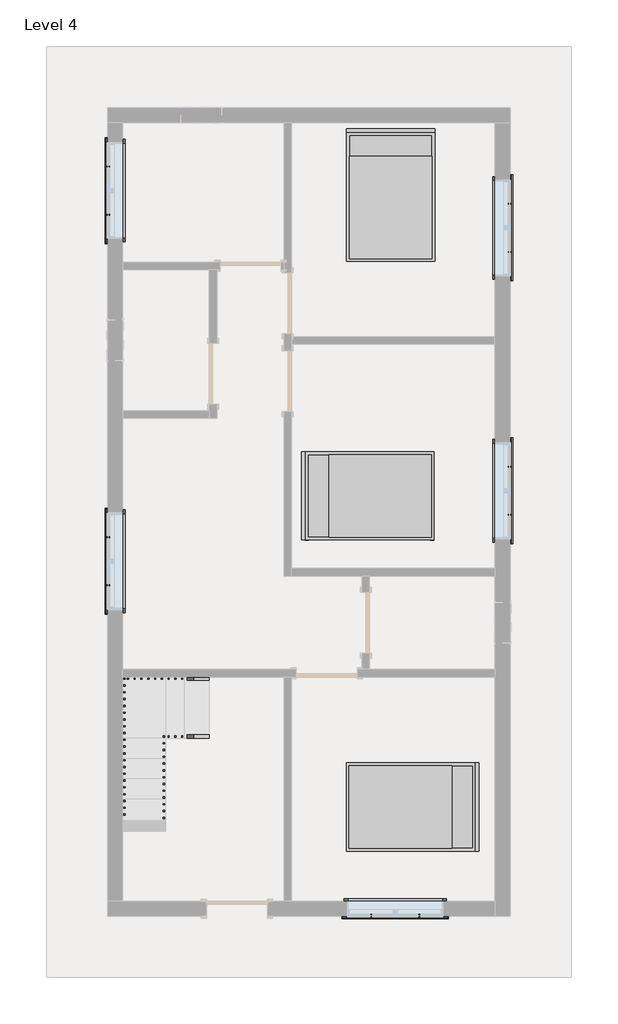
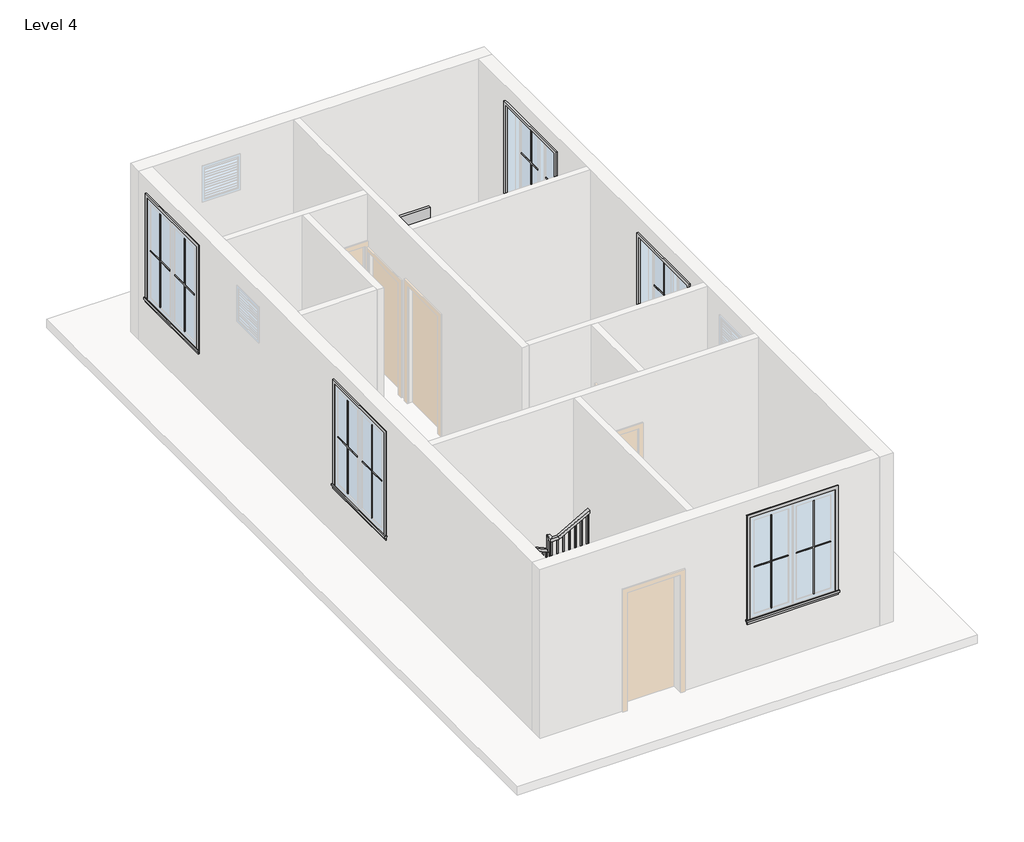
# One storey, part 2 of 2: 20 proxies, 3 furniture elements, 2 railings.
"""IFC4 building model written with IfcOpenShell, lengths in millimetres."""

from ifc_helpers import new_model, si_unit, frame, origin, place, context, project, spatial, polyline, outline, extrude, faceted_brep, transform, mapped, element, save
from components import muntin_pattern_2x2_muntin_pattern_2x2_bff912c5, muntin_pattern_2x2_muntin_pattern_2x2_c2194282, trim_window_exterior_flat_with_sill_e04b3088, trim_window_interior_flat_picture_frame_2a7685fe, bed_17739_bed_17739_15c61121

model = new_model("IFC4")

# Units and contexts
model_context = context("Model", 3, world=origin())
ifc_project = project(units=[si_unit("LENGTHUNIT", "METRE", prefix="MILLI")], contexts=[model_context])

# Site, building, storey
site = spatial("IfcSite", under=ifc_project)
building = spatial("IfcBuilding", under=site)
storey = spatial("IfcBuildingStorey", under=building, Name="Level 4", Elevation=6400.8)

# Proxies
placement = place(None, origin())
muntin_pattern_2x2_muntin_pattern_2x2_shape = muntin_pattern_2x2_muntin_pattern_2x2_bff912c5(model_context)
element("IfcBuildingElementProxy", 1, Name="Muntin Pattern_2x2 : Muntin Pattern_2x2", ObjectType="Muntin Pattern_2x2 : Muntin Pattern_2x2", at=placement, inside=storey, context=model_context, shape_type="MappedRepresentation", body=[
    mapped(muntin_pattern_2x2_muntin_pattern_2x2_shape, transform((-4261.9639285, 4584.2694249, 7385.05), x_axis=(0.0, 1.0, 0.0), y_axis=(-1.0, 0.0, 0.0), z_axis=(0.0, 0.0, 1.0))),
])
element("IfcBuildingElementProxy", 2, Name="Muntin Pattern_2x2 : Muntin Pattern_2x2", ObjectType="Muntin Pattern_2x2 : Muntin Pattern_2x2", at=placement, inside=storey, context=model_context, shape_type="MappedRepresentation", body=[
    mapped(muntin_pattern_2x2_muntin_pattern_2x2_shape, transform((1751.4860715, 4746.1944249, 7385.05), x_axis=(0.0, -1.0, 0.0), y_axis=(1.0, 0.0, 0.0), z_axis=(0.0, 0.0, 1.0))),
])
element("IfcBuildingElementProxy", 3, Name="Muntin Pattern_2x2 : Muntin Pattern_2x2", ObjectType="Muntin Pattern_2x2 : Muntin Pattern_2x2", at=placement, inside=storey, context=model_context, shape_type="MappedRepresentation", body=[
    mapped(muntin_pattern_2x2_muntin_pattern_2x2_shape, transform((-4261.9639285, -962.4555751, 7385.05), x_axis=(0.0, 1.0, 0.0), y_axis=(-1.0, 0.0, 0.0), z_axis=(0.0, 0.0, 1.0))),
])
element("IfcBuildingElementProxy", 4, Name="Muntin Pattern_2x2 : Muntin Pattern_2x2", ObjectType="Muntin Pattern_2x2 : Muntin Pattern_2x2", at=placement, inside=storey, context=model_context, shape_type="MappedRepresentation", body=[
    mapped(muntin_pattern_2x2_muntin_pattern_2x2_shape, transform((1751.4860715, 812.3694249, 7385.05), x_axis=(0.0, -1.0, 0.0), y_axis=(1.0, 0.0, 0.0), z_axis=(0.0, 0.0, 1.0))),
])
element("IfcBuildingElementProxy", 5, Name="Muntin Pattern_2x2 : Muntin Pattern_2x2", ObjectType="Muntin Pattern_2x2 : Muntin Pattern_2x2", at=placement, inside=storey, context=model_context, shape_type="MappedRepresentation", body=[
    mapped(muntin_pattern_2x2_muntin_pattern_2x2_shape, transform((397.3485715, -5907.5180751, 7385.05), x_axis=(-1.0, 0.0, 0.0), y_axis=(0.0, -1.0, 0.0), z_axis=(0.0, 0.0, 1.0))),
])
muntin_pattern_2x2_muntin_pattern_2x2_2_shape = muntin_pattern_2x2_muntin_pattern_2x2_c2194282(model_context)
element("IfcBuildingElementProxy", 6, Name="Muntin Pattern_2x2 : Muntin Pattern_2x2", ObjectType="Muntin Pattern_2x2 : Muntin Pattern_2x2", at=placement, inside=storey, context=model_context, shape_type="MappedRepresentation", body=[
    mapped(muntin_pattern_2x2_muntin_pattern_2x2_2_shape, transform((-4261.9639285, 5304.9944249, 7385.05), x_axis=(0.0, -1.0, 0.0), y_axis=(1.0, 0.0, 0.0), z_axis=(0.0, 0.0, 1.0))),
])
element("IfcBuildingElementProxy", 7, Name="Muntin Pattern_2x2 : Muntin Pattern_2x2", ObjectType="Muntin Pattern_2x2 : Muntin Pattern_2x2", at=placement, inside=storey, context=model_context, shape_type="MappedRepresentation", body=[
    mapped(muntin_pattern_2x2_muntin_pattern_2x2_2_shape, transform((1751.4860715, 4025.4694249, 7385.05), x_axis=(0.0, 1.0, 0.0), y_axis=(-1.0, 0.0, 0.0), z_axis=(0.0, 0.0, 1.0))),
])
element("IfcBuildingElementProxy", 8, Name="Muntin Pattern_2x2 : Muntin Pattern_2x2", ObjectType="Muntin Pattern_2x2 : Muntin Pattern_2x2", at=placement, inside=storey, context=model_context, shape_type="MappedRepresentation", body=[
    mapped(muntin_pattern_2x2_muntin_pattern_2x2_2_shape, transform((-4261.9639285, -241.7305751, 7385.05), x_axis=(0.0, -1.0, 0.0), y_axis=(1.0, 0.0, 0.0), z_axis=(0.0, 0.0, 1.0))),
])
element("IfcBuildingElementProxy", 9, Name="Muntin Pattern_2x2 : Muntin Pattern_2x2", ObjectType="Muntin Pattern_2x2 : Muntin Pattern_2x2", at=placement, inside=storey, context=model_context, shape_type="MappedRepresentation", body=[
    mapped(muntin_pattern_2x2_muntin_pattern_2x2_2_shape, transform((1751.4860715, 91.6444249, 7385.05), x_axis=(0.0, 1.0, 0.0), y_axis=(-1.0, 0.0, 0.0), z_axis=(0.0, 0.0, 1.0))),
])
element("IfcBuildingElementProxy", 10, Name="Muntin Pattern_2x2 : Muntin Pattern_2x2", ObjectType="Muntin Pattern_2x2 : Muntin Pattern_2x2", at=placement, inside=storey, context=model_context, shape_type="MappedRepresentation", body=[
    mapped(muntin_pattern_2x2_muntin_pattern_2x2_2_shape, transform((-323.3764285, -5907.5180751, 7385.05), x_axis=(1.0, 0.0, 0.0), y_axis=(0.0, 1.0, 0.0), z_axis=(0.0, 0.0, 1.0))),
])
trim_window_exterior_flat_with_sill_shape = trim_window_exterior_flat_with_sill_e04b3088(model_context)
element("IfcBuildingElementProxy", 11, Name="Trim-Window-Exterior-Flat : with Sill", ObjectType="Trim-Window-Exterior-Flat : with Sill", at=placement, inside=storey, context=model_context, shape_type="MappedRepresentation", body=[
    mapped(trim_window_exterior_flat_with_sill_shape, transform((-4271.4889285, 4944.6319249, 9144.0), x_axis=(0.0, -1.0, 0.0), y_axis=(0.0, 0.0, 1.0), z_axis=(-1.0, 0.0, 0.0))),
])
element("IfcBuildingElementProxy", 12, Name="Trim-Window-Exterior-Flat : with Sill", ObjectType="Trim-Window-Exterior-Flat : with Sill", at=placement, inside=storey, context=model_context, shape_type="MappedRepresentation", body=[
    mapped(trim_window_exterior_flat_with_sill_shape, transform((1761.0110715, 4385.8319249, 9144.0), x_axis=(0.0, 1.0, 0.0), y_axis=(0.0, 0.0, 1.0), z_axis=(1.0, 0.0, 0.0))),
])
element("IfcBuildingElementProxy", 13, Name="Trim-Window-Exterior-Flat : with Sill", ObjectType="Trim-Window-Exterior-Flat : with Sill", at=placement, inside=storey, context=model_context, shape_type="MappedRepresentation", body=[
    mapped(trim_window_exterior_flat_with_sill_shape, transform((-4271.4889285, -602.0930751, 9144.0), x_axis=(0.0, -1.0, 0.0), y_axis=(0.0, 0.0, 1.0), z_axis=(-1.0, 0.0, 0.0))),
])
element("IfcBuildingElementProxy", 14, Name="Trim-Window-Exterior-Flat : with Sill", ObjectType="Trim-Window-Exterior-Flat : with Sill", at=placement, inside=storey, context=model_context, shape_type="MappedRepresentation", body=[
    mapped(trim_window_exterior_flat_with_sill_shape, transform((1761.0110715, 452.0069249, 9144.0), x_axis=(0.0, 1.0, 0.0), y_axis=(0.0, 0.0, 1.0), z_axis=(1.0, 0.0, 0.0))),
])
element("IfcBuildingElementProxy", 15, Name="Trim-Window-Exterior-Flat : with Sill", ObjectType="Trim-Window-Exterior-Flat : with Sill", at=placement, inside=storey, context=model_context, shape_type="MappedRepresentation", body=[
    mapped(trim_window_exterior_flat_with_sill_shape, transform((36.9860715, -5917.0430751, 9144.0), x_axis=(1.0, 0.0, 0.0), y_axis=(0.0, 0.0, 1.0), z_axis=(0.0, -1.0, 0.0))),
])
trim_window_interior_flat_picture_frame_shape = trim_window_interior_flat_picture_frame_2a7685fe(model_context)
element("IfcBuildingElementProxy", 16, Name="Trim-Window-Interior-Flat : Picture Frame", ObjectType="Trim-Window-Interior-Flat : Picture Frame", at=placement, inside=storey, context=model_context, shape_type="MappedRepresentation", body=[
    mapped(trim_window_interior_flat_picture_frame_shape, transform((-4042.8889285, 4944.6319249, 9144.0), x_axis=(0.0, 1.0, 0.0), y_axis=(0.0, 0.0, 1.0), z_axis=(1.0, 0.0, 0.0))),
])
element("IfcBuildingElementProxy", 17, Name="Trim-Window-Interior-Flat : Picture Frame", ObjectType="Trim-Window-Interior-Flat : Picture Frame", at=placement, inside=storey, context=model_context, shape_type="MappedRepresentation", body=[
    mapped(trim_window_interior_flat_picture_frame_shape, transform((1532.4110715, 4385.8319249, 9144.0), x_axis=(0.0, -1.0, 0.0), y_axis=(0.0, 0.0, 1.0), z_axis=(-1.0, 0.0, 0.0))),
])
element("IfcBuildingElementProxy", 18, Name="Trim-Window-Interior-Flat : Picture Frame", ObjectType="Trim-Window-Interior-Flat : Picture Frame", at=placement, inside=storey, context=model_context, shape_type="MappedRepresentation", body=[
    mapped(trim_window_interior_flat_picture_frame_shape, transform((-4042.8889285, -602.0930751, 9144.0), x_axis=(0.0, 1.0, 0.0), y_axis=(0.0, 0.0, 1.0), z_axis=(1.0, 0.0, 0.0))),
])
element("IfcBuildingElementProxy", 19, Name="Trim-Window-Interior-Flat : Picture Frame", ObjectType="Trim-Window-Interior-Flat : Picture Frame", at=placement, inside=storey, context=model_context, shape_type="MappedRepresentation", body=[
    mapped(trim_window_interior_flat_picture_frame_shape, transform((1532.4110715, 452.0069249, 9144.0), x_axis=(0.0, -1.0, 0.0), y_axis=(0.0, 0.0, 1.0), z_axis=(-1.0, 0.0, 0.0))),
])
element("IfcBuildingElementProxy", 20, Name="Trim-Window-Interior-Flat : Picture Frame", ObjectType="Trim-Window-Interior-Flat : Picture Frame", at=placement, inside=storey, context=model_context, shape_type="MappedRepresentation", body=[
    mapped(trim_window_interior_flat_picture_frame_shape, transform((36.9860715, -5688.4430751, 9144.0), x_axis=(-1.0, 0.0, 0.0), y_axis=(0.0, 0.0, 1.0), z_axis=(0.0, 1.0, 0.0))),
])

# Furniture
bed_17739_bed_17739_shape = bed_17739_bed_17739_15c61121(model_context)
element("IfcFurniture", 21, ObjectType="Bed_17739 : Bed_17739", at=placement, inside=storey, context=model_context, shape_type="MappedRepresentation", body=[
    mapped(bed_17739_bed_17739_shape, transform((-29.6889285, 4852.5569249, 6400.8), x_axis=(1.0, 0.0, 0.0), y_axis=(0.0, 1.0, 0.0), z_axis=(0.0, 0.0, 1.0))),
])
element("IfcFurniture", 22, ObjectType="Bed_17739 : Bed_17739", at=placement, inside=storey, context=model_context, shape_type="MappedRepresentation", body=[
    mapped(bed_17739_bed_17739_shape, transform((-347.1889285, 375.8069249, 6400.8), x_axis=(0.0, 1.0, 0.0), y_axis=(-1.0, 0.0, 0.0), z_axis=(0.0, 0.0, 1.0))),
])
element("IfcFurniture", 23, ObjectType="Bed_17739 : Bed_17739", at=placement, inside=storey, context=model_context, shape_type="MappedRepresentation", body=[
    mapped(bed_17739_bed_17739_shape, transform((275.1110715, -4278.7430751, 6400.8), x_axis=(0.0, -1.0, 0.0), y_axis=(1.0, 0.0, 0.0), z_axis=(0.0, 0.0, 1.0))),
])

# Railings
element("IfcRailing", 24, ObjectType="Handrail - Rectangular", at=placement, inside=storey, context=model_context, shape_type="SolidModel", body=[
    faceted_brep([(-2747.4889285, -2386.4430751, 7484.5333333), (-2747.4889285, -2386.4430751, 7427.3271159), (-2747.4889285, -2335.6430751, 7427.3271159), (-2747.4889285, -2335.6430751, 7484.5333333), (-3396.0267484, -2386.4430751, 7820.3457967), (-3408.3987558, -2386.4430751, 7769.5457967), (-3408.3987558, -2335.6430751, 7769.5457967), (-3396.0267484, -2335.6430751, 7820.3457967), (-3992.0889285, -2386.4430751, 7820.3457967), (-3992.0889285, -2386.4430751, 7769.5457967), (-4042.8889285, -2335.6430751, 7769.5457967), (-4042.8889285, -2335.6430751, 7820.3457967), (-3992.0889285, -2940.1628326, 7820.3457967), (-3992.0889285, -2953.3285634, 7769.5457967), (-4042.8889285, -2953.3285634, 7769.5457967), (-4042.8889285, -2940.1628326, 7820.3457967), (-3992.0889285, -5061.9991591, 8999.3618165), (-3992.0889285, -5075.1648899, 8948.5618165), (-4042.8889285, -5075.1648899, 8948.5618165), (-4042.8889285, -5061.9991591, 8999.3618165), (-3992.0889285, -5637.6430751, 8999.3618165), (-3992.0889285, -5637.6430751, 8948.5618165), (-4042.8889285, -5688.4430751, 8948.5618165), (-4042.8889285, -5688.4430751, 8999.3618165), (-3418.001852, -5637.6430751, 8999.3618165), (-3404.8062484, -5637.6430751, 8948.5618165), (-3404.8062484, -5688.4430751, 8948.5618165), (-3418.001852, -5688.4430751, 8999.3618165), (-2793.6303845, -5637.6430751, 9347.2), (-2793.6303845, -5688.4430751, 9347.2), (-2793.6303845, -5688.4430751, 9289.0487115), (-2793.6303845, -5637.6430751, 9289.0487115)], [[[0, 1, 2, 3]], [[1, 0, 4, 5]], [[2, 1, 5, 6]], [[3, 2, 6, 7]], [[0, 3, 7, 4]], [[5, 4, 8, 9]], [[6, 5, 9, 10]], [[7, 6, 10, 11]], [[4, 7, 11, 8]], [[9, 8, 12, 13]], [[10, 9, 13, 14]], [[11, 10, 14, 15]], [[8, 11, 15, 12]], [[13, 12, 16, 17]], [[14, 13, 17, 18]], [[15, 14, 18, 19]], [[12, 15, 19, 16]], [[17, 16, 20, 21]], [[18, 17, 21, 22]], [[19, 18, 22, 23]], [[16, 19, 23, 20]], [[21, 20, 24, 25]], [[22, 21, 25, 26]], [[23, 22, 26, 27]], [[20, 23, 27, 24]], [[28, 29, 30, 31]], [[25, 24, 28, 31]], [[26, 25, 31, 30]], [[27, 26, 30, 29]], [[24, 27, 29, 28]]]),
    extrude(outline(polyline([(9291.7598207, -2788.7639285), (9281.1470401, -2807.8139285), (8263.4666667, -2807.8139285), (8263.4666667, -2788.7639285), (9291.7598207, -2788.7639285)])), frame((0.0, -5672.5680751, 0.0), z_axis=(0.0, 1.0, 0.0), x_axis=(0.0, 0.0, 1.0)), (0.0, 0.0, 1.0), 19.05),
    extrude(outline(polyline([(9235.1583242, -2890.3639285), (9224.5455436, -2909.4139285), (8263.4666667, -2909.4139285), (8263.4666667, -2890.3639285), (9235.1583242, -2890.3639285)])), frame((0.0, -5672.5680751, 0.0), z_axis=(0.0, 1.0, 0.0), x_axis=(0.0, 0.0, 1.0)), (0.0, 0.0, 1.0), 19.05),
    extrude(outline(polyline([(9178.5568277, -2991.9639285), (9167.9440471, -3011.0139285), (8263.4666667, -3011.0139285), (8263.4666667, -2991.9639285), (9178.5568277, -2991.9639285)])), frame((0.0, -5672.5680751, 0.0), z_axis=(0.0, 1.0, 0.0), x_axis=(0.0, 0.0, 1.0)), (0.0, 0.0, 1.0), 19.05),
    extrude(outline(polyline([(9121.9553312, -3093.5639285), (9111.3425506, -3112.6139285), (8263.4666667, -3112.6139285), (8263.4666667, -3093.5639285), (9121.9553312, -3093.5639285)])), frame((0.0, -5672.5680751, 0.0), z_axis=(0.0, 1.0, 0.0), x_axis=(0.0, 0.0, 1.0)), (0.0, 0.0, 1.0), 19.05),
    extrude(outline(polyline([(9065.3538346, -3195.1639285), (9054.7410541, -3214.2139285), (8094.1333333, -3214.2139285), (8094.1333333, -3195.1639285), (9065.3538346, -3195.1639285)])), frame((0.0, -5672.5680751, 0.0), z_axis=(0.0, 1.0, 0.0), x_axis=(0.0, 0.0, 1.0)), (0.0, 0.0, 1.0), 19.05),
    extrude(outline(polyline([(9008.7523381, -3296.7639285), (8998.1395575, -3315.8139285), (8094.1333333, -3315.8139285), (8094.1333333, -3296.7639285), (9008.7523381, -3296.7639285)])), frame((0.0, -5672.5680751, 0.0), z_axis=(0.0, 1.0, 0.0), x_axis=(0.0, 0.0, 1.0)), (0.0, 0.0, 1.0), 19.05),
    extrude(outline(polyline([(8952.1508416, -3398.3639285), (8941.538061, -3417.4139285), (7924.8, -3417.4139285), (7924.8, -3398.3639285), (8952.1508416, -3398.3639285)])), frame((0.0, -5672.5680751, 0.0), z_axis=(0.0, 1.0, 0.0), x_axis=(0.0, 0.0, 1.0)), (0.0, 0.0, 1.0), 19.05),
    extrude(outline(polyline([(-3519.0139285, -5672.5680751), (-3519.0139285, -5653.5180751), (-3499.9639285, -5653.5180751), (-3499.9639285, -5672.5680751), (-3519.0139285, -5672.5680751)])), frame((0.0, 0.0, 7924.8), z_axis=(0.0, 0.0, 1.0), x_axis=(1.0, 0.0, 0.0)), (0.0, 0.0, 1.0), 1023.7618165),
    extrude(outline(polyline([(-3620.6139285, -5672.5680751), (-3620.6139285, -5653.5180751), (-3601.5639285, -5653.5180751), (-3601.5639285, -5672.5680751), (-3620.6139285, -5672.5680751)])), frame((0.0, 0.0, 7924.8), z_axis=(0.0, 0.0, 1.0), x_axis=(1.0, 0.0, 0.0)), (0.0, 0.0, 1.0), 1023.7618165),
    extrude(outline(polyline([(-3722.2139285, -5672.5680751), (-3722.2139285, -5653.5180751), (-3703.1639285, -5653.5180751), (-3703.1639285, -5672.5680751), (-3722.2139285, -5672.5680751)])), frame((0.0, 0.0, 7924.8), z_axis=(0.0, 0.0, 1.0), x_axis=(1.0, 0.0, 0.0)), (0.0, 0.0, 1.0), 1023.7618165),
    extrude(outline(polyline([(-3823.8139285, -5672.5680751), (-3823.8139285, -5653.5180751), (-3804.7639285, -5653.5180751), (-3804.7639285, -5672.5680751), (-3823.8139285, -5672.5680751)])), frame((0.0, 0.0, 7924.8), z_axis=(0.0, 0.0, 1.0), x_axis=(1.0, 0.0, 0.0)), (0.0, 0.0, 1.0), 1023.7618165),
    extrude(outline(polyline([(-3925.4139285, -5672.5680751), (-3925.4139285, -5653.5180751), (-3906.3639285, -5653.5180751), (-3906.3639285, -5672.5680751), (-3925.4139285, -5672.5680751)])), frame((0.0, 0.0, 7924.8), z_axis=(0.0, 0.0, 1.0), x_axis=(1.0, 0.0, 0.0)), (0.0, 0.0, 1.0), 1023.7618165),
    extrude(outline(polyline([(-4027.0139285, -5602.7180751), (-4007.9639285, -5602.7180751), (-4007.9639285, -5621.7680751), (-4027.0139285, -5621.7680751), (-4027.0139285, -5602.7180751)])), frame((0.0, 0.0, 7924.8), z_axis=(0.0, 0.0, 1.0), x_axis=(1.0, 0.0, 0.0)), (0.0, 0.0, 1.0), 1023.7618165),
    extrude(outline(polyline([(-4027.0139285, -5501.1180751), (-4007.9639285, -5501.1180751), (-4007.9639285, -5520.1680751), (-4027.0139285, -5520.1680751), (-4027.0139285, -5501.1180751)])), frame((0.0, 0.0, 7924.8), z_axis=(0.0, 0.0, 1.0), x_axis=(1.0, 0.0, 0.0)), (0.0, 0.0, 1.0), 1023.7618165),
    extrude(outline(polyline([(-4027.0139285, -5399.5180751), (-4007.9639285, -5399.5180751), (-4007.9639285, -5418.5680751), (-4027.0139285, -5418.5680751), (-4027.0139285, -5399.5180751)])), frame((0.0, 0.0, 7924.8), z_axis=(0.0, 0.0, 1.0), x_axis=(1.0, 0.0, 0.0)), (0.0, 0.0, 1.0), 1023.7618165),
    extrude(outline(polyline([(-4027.0139285, -5297.9180751), (-4007.9639285, -5297.9180751), (-4007.9639285, -5316.9680751), (-4027.0139285, -5316.9680751), (-4027.0139285, -5297.9180751)])), frame((0.0, 0.0, 7924.8), z_axis=(0.0, 0.0, 1.0), x_axis=(1.0, 0.0, 0.0)), (0.0, 0.0, 1.0), 1023.7618165),
    extrude(outline(polyline([(-4027.0139285, -5196.3180751), (-4007.9639285, -5196.3180751), (-4007.9639285, -5215.3680751), (-4027.0139285, -5215.3680751), (-4027.0139285, -5196.3180751)])), frame((0.0, 0.0, 7924.8), z_axis=(0.0, 0.0, 1.0), x_axis=(1.0, 0.0, 0.0)), (0.0, 0.0, 1.0), 1023.7618165),
    extrude(outline(polyline([(-4027.0139285, -5094.7180751), (-4007.9639285, -5094.7180751), (-4007.9639285, -5113.7680751), (-4027.0139285, -5113.7680751), (-4027.0139285, -5094.7180751)])), frame((0.0, 0.0, 7924.8), z_axis=(0.0, 0.0, 1.0), x_axis=(1.0, 0.0, 0.0)), (0.0, 0.0, 1.0), 1023.7618165),
    extrude(outline(polyline([(-5012.1680751, 8913.5571119), (-4993.1180751, 8902.9718208), (-4993.1180751, 7924.8), (-5012.1680751, 7924.8), (-5012.1680751, 8913.5571119)])), frame((-4027.0139285, 0.0, 0.0), z_axis=(1.0, 0.0, 0.0), x_axis=(0.0, 1.0, 0.0)), (0.0, 0.0, 1.0), 19.05),
    extrude(outline(polyline([(-4910.5680751, 8857.1022261), (-4891.5180751, 8846.516935), (-4891.5180751, 7924.8), (-4910.5680751, 7924.8), (-4910.5680751, 8857.1022261)])), frame((-4027.0139285, 0.0, 0.0), z_axis=(1.0, 0.0, 0.0), x_axis=(0.0, 1.0, 0.0)), (0.0, 0.0, 1.0), 19.05),
    extrude(outline(polyline([(-4808.9680751, 8800.6473402), (-4789.9180751, 8790.0620491), (-4789.9180751, 7924.8), (-4808.9680751, 7924.8), (-4808.9680751, 8800.6473402)])), frame((-4027.0139285, 0.0, 0.0), z_axis=(1.0, 0.0, 0.0), x_axis=(0.0, 1.0, 0.0)), (0.0, 0.0, 1.0), 19.05),
    extrude(outline(polyline([(-4707.3680751, 8744.0358332), (-4688.3180751, 8733.4505421), (-4688.3180751, 7755.4666667), (-4707.3680751, 7755.4666667), (-4707.3680751, 8744.0358332)])), frame((-4027.0139285, 0.0, 0.0), z_axis=(1.0, 0.0, 0.0), x_axis=(0.0, 1.0, 0.0)), (0.0, 0.0, 1.0), 19.05),
    extrude(outline(polyline([(-4605.7680751, 8687.5809474), (-4586.7180751, 8676.9956563), (-4586.7180751, 7755.4666667), (-4605.7680751, 7755.4666667), (-4605.7680751, 8687.5809474)])), frame((-4027.0139285, 0.0, 0.0), z_axis=(1.0, 0.0, 0.0), x_axis=(0.0, 1.0, 0.0)), (0.0, 0.0, 1.0), 19.05),
    extrude(outline(polyline([(-4504.1680751, 8631.1260615), (-4485.1180751, 8620.5407704), (-4485.1180751, 7755.4666667), (-4504.1680751, 7755.4666667), (-4504.1680751, 8631.1260615)])), frame((-4027.0139285, 0.0, 0.0), z_axis=(1.0, 0.0, 0.0), x_axis=(0.0, 1.0, 0.0)), (0.0, 0.0, 1.0), 19.05),
    extrude(outline(polyline([(-4402.5680751, 8574.7024999), (-4383.5180751, 8564.1172088), (-4383.5180751, 7586.1333333), (-4402.5680751, 7586.1333333), (-4402.5680751, 8574.7024999)])), frame((-4027.0139285, 0.0, 0.0), z_axis=(1.0, 0.0, 0.0), x_axis=(0.0, 1.0, 0.0)), (0.0, 0.0, 1.0), 19.05),
    extrude(outline(polyline([(-4300.9680751, 8518.247614), (-4281.9180751, 8507.6623229), (-4281.9180751, 7586.1333333), (-4300.9680751, 7586.1333333), (-4300.9680751, 8518.247614)])), frame((-4027.0139285, 0.0, 0.0), z_axis=(1.0, 0.0, 0.0), x_axis=(0.0, 1.0, 0.0)), (0.0, 0.0, 1.0), 19.05),
    extrude(outline(polyline([(-4199.3680751, 8461.7927282), (-4180.3180751, 8451.2074371), (-4180.3180751, 7586.1333333), (-4199.3680751, 7586.1333333), (-4199.3680751, 8461.7927282)])), frame((-4027.0139285, 0.0, 0.0), z_axis=(1.0, 0.0, 0.0), x_axis=(0.0, 1.0, 0.0)), (0.0, 0.0, 1.0), 19.05),
    extrude(outline(polyline([(-4097.7680751, 8405.3691666), (-4078.7180751, 8394.7838755), (-4078.7180751, 7416.8), (-4097.7680751, 7416.8), (-4097.7680751, 8405.3691666)])), frame((-4027.0139285, 0.0, 0.0), z_axis=(1.0, 0.0, 0.0), x_axis=(0.0, 1.0, 0.0)), (0.0, 0.0, 1.0), 19.05),
    extrude(outline(polyline([(-3996.1680751, 8348.9142807), (-3977.1180751, 8338.3289896), (-3977.1180751, 7416.8), (-3996.1680751, 7416.8), (-3996.1680751, 8348.9142807)])), frame((-4027.0139285, 0.0, 0.0), z_axis=(1.0, 0.0, 0.0), x_axis=(0.0, 1.0, 0.0)), (0.0, 0.0, 1.0), 19.05),
    extrude(outline(polyline([(-3894.5680751, 8292.4593949), (-3875.5180751, 8281.8741038), (-3875.5180751, 7416.8), (-3894.5680751, 7416.8), (-3894.5680751, 8292.4593949)])), frame((-4027.0139285, 0.0, 0.0), z_axis=(1.0, 0.0, 0.0), x_axis=(0.0, 1.0, 0.0)), (0.0, 0.0, 1.0), 19.05),
    extrude(outline(polyline([(-3792.9680751, 8236.0358332), (-3773.9180751, 8225.4505421), (-3773.9180751, 7247.4666667), (-3792.9680751, 7247.4666667), (-3792.9680751, 8236.0358332)])), frame((-4027.0139285, 0.0, 0.0), z_axis=(1.0, 0.0, 0.0), x_axis=(0.0, 1.0, 0.0)), (0.0, 0.0, 1.0), 19.05),
    extrude(outline(polyline([(-3691.3680751, 8179.5809474), (-3672.3180751, 8168.9956563), (-3672.3180751, 7247.4666667), (-3691.3680751, 7247.4666667), (-3691.3680751, 8179.5809474)])), frame((-4027.0139285, 0.0, 0.0), z_axis=(1.0, 0.0, 0.0), x_axis=(0.0, 1.0, 0.0)), (0.0, 0.0, 1.0), 19.05),
    extrude(outline(polyline([(-3589.7680751, 8123.1260615), (-3570.7180751, 8112.5407704), (-3570.7180751, 7247.4666667), (-3589.7680751, 7247.4666667), (-3589.7680751, 8123.1260615)])), frame((-4027.0139285, 0.0, 0.0), z_axis=(1.0, 0.0, 0.0), x_axis=(0.0, 1.0, 0.0)), (0.0, 0.0, 1.0), 19.05),
    extrude(outline(polyline([(-3488.1680751, 8066.7024999), (-3469.1180751, 8056.1172088), (-3469.1180751, 7078.1333333), (-3488.1680751, 7078.1333333), (-3488.1680751, 8066.7024999)])), frame((-4027.0139285, 0.0, 0.0), z_axis=(1.0, 0.0, 0.0), x_axis=(0.0, 1.0, 0.0)), (0.0, 0.0, 1.0), 19.05),
    extrude(outline(polyline([(-3386.5680751, 8010.247614), (-3367.5180751, 7999.6623229), (-3367.5180751, 7078.1333333), (-3386.5680751, 7078.1333333), (-3386.5680751, 8010.247614)])), frame((-4027.0139285, 0.0, 0.0), z_axis=(1.0, 0.0, 0.0), x_axis=(0.0, 1.0, 0.0)), (0.0, 0.0, 1.0), 19.05),
    extrude(outline(polyline([(-3284.9680751, 7953.7927282), (-3265.9180751, 7943.2074371), (-3265.9180751, 7078.1333333), (-3284.9680751, 7078.1333333), (-3284.9680751, 7953.7927282)])), frame((-4027.0139285, 0.0, 0.0), z_axis=(1.0, 0.0, 0.0), x_axis=(0.0, 1.0, 0.0)), (0.0, 0.0, 1.0), 19.05),
    extrude(outline(polyline([(-3183.3680751, 7897.3691666), (-3164.3180751, 7886.7838755), (-3164.3180751, 6908.8), (-3183.3680751, 6908.8), (-3183.3680751, 7897.3691666)])), frame((-4027.0139285, 0.0, 0.0), z_axis=(1.0, 0.0, 0.0), x_axis=(0.0, 1.0, 0.0)), (0.0, 0.0, 1.0), 19.05),
    extrude(outline(polyline([(-3081.7680751, 7840.9142807), (-3062.7180751, 7830.3289896), (-3062.7180751, 6908.8), (-3081.7680751, 6908.8), (-3081.7680751, 7840.9142807)])), frame((-4027.0139285, 0.0, 0.0), z_axis=(1.0, 0.0, 0.0), x_axis=(0.0, 1.0, 0.0)), (0.0, 0.0, 1.0), 19.05),
    extrude(outline(polyline([(-2980.1680751, 7784.4593949), (-2961.1180751, 7773.8741038), (-2961.1180751, 6908.8), (-2980.1680751, 6908.8), (-2980.1680751, 7784.4593949)])), frame((-4027.0139285, 0.0, 0.0), z_axis=(1.0, 0.0, 0.0), x_axis=(0.0, 1.0, 0.0)), (0.0, 0.0, 1.0), 19.05),
    extrude(outline(polyline([(-4027.0139285, -2859.5180751), (-4007.9639285, -2859.5180751), (-4007.9639285, -2878.5680751), (-4027.0139285, -2878.5680751), (-4027.0139285, -2859.5180751)])), frame((0.0, 0.0, 6908.8), z_axis=(0.0, 0.0, 1.0), x_axis=(1.0, 0.0, 0.0)), (0.0, 0.0, 1.0), 860.7457967),
    extrude(outline(polyline([(-4027.0139285, -2757.9180751), (-4007.9639285, -2757.9180751), (-4007.9639285, -2776.9680751), (-4027.0139285, -2776.9680751), (-4027.0139285, -2757.9180751)])), frame((0.0, 0.0, 6908.8), z_axis=(0.0, 0.0, 1.0), x_axis=(1.0, 0.0, 0.0)), (0.0, 0.0, 1.0), 860.7457967),
    extrude(outline(polyline([(-4027.0139285, -2656.3180751), (-4007.9639285, -2656.3180751), (-4007.9639285, -2675.3680751), (-4027.0139285, -2675.3680751), (-4027.0139285, -2656.3180751)])), frame((0.0, 0.0, 6908.8), z_axis=(0.0, 0.0, 1.0), x_axis=(1.0, 0.0, 0.0)), (0.0, 0.0, 1.0), 860.7457967),
    extrude(outline(polyline([(-4027.0139285, -2554.7180751), (-4007.9639285, -2554.7180751), (-4007.9639285, -2573.7680751), (-4027.0139285, -2573.7680751), (-4027.0139285, -2554.7180751)])), frame((0.0, 0.0, 6908.8), z_axis=(0.0, 0.0, 1.0), x_axis=(1.0, 0.0, 0.0)), (0.0, 0.0, 1.0), 860.7457967),
    extrude(outline(polyline([(-4027.0139285, -2453.1180751), (-4007.9639285, -2453.1180751), (-4007.9639285, -2472.1680751), (-4027.0139285, -2472.1680751), (-4027.0139285, -2453.1180751)])), frame((0.0, 0.0, 6908.8), z_axis=(0.0, 0.0, 1.0), x_axis=(1.0, 0.0, 0.0)), (0.0, 0.0, 1.0), 860.7457967),
    extrude(outline(polyline([(-3957.1639285, -2351.5180751), (-3957.1639285, -2370.5680751), (-3976.2139285, -2370.5680751), (-3976.2139285, -2351.5180751), (-3957.1639285, -2351.5180751)])), frame((0.0, 0.0, 6908.8), z_axis=(0.0, 0.0, 1.0), x_axis=(1.0, 0.0, 0.0)), (0.0, 0.0, 1.0), 860.7457967),
    extrude(outline(polyline([(-3855.5639285, -2351.5180751), (-3855.5639285, -2370.5680751), (-3874.6139285, -2370.5680751), (-3874.6139285, -2351.5180751), (-3855.5639285, -2351.5180751)])), frame((0.0, 0.0, 6908.8), z_axis=(0.0, 0.0, 1.0), x_axis=(1.0, 0.0, 0.0)), (0.0, 0.0, 1.0), 860.7457967),
    extrude(outline(polyline([(-3753.9639285, -2351.5180751), (-3753.9639285, -2370.5680751), (-3773.0139285, -2370.5680751), (-3773.0139285, -2351.5180751), (-3753.9639285, -2351.5180751)])), frame((0.0, 0.0, 6908.8), z_axis=(0.0, 0.0, 1.0), x_axis=(1.0, 0.0, 0.0)), (0.0, 0.0, 1.0), 860.7457967),
    extrude(outline(polyline([(-3652.3639285, -2351.5180751), (-3652.3639285, -2370.5680751), (-3671.4139285, -2370.5680751), (-3671.4139285, -2351.5180751), (-3652.3639285, -2351.5180751)])), frame((0.0, 0.0, 6908.8), z_axis=(0.0, 0.0, 1.0), x_axis=(1.0, 0.0, 0.0)), (0.0, 0.0, 1.0), 860.7457967),
    extrude(outline(polyline([(-3550.7639285, -2351.5180751), (-3550.7639285, -2370.5680751), (-3569.8139285, -2370.5680751), (-3569.8139285, -2351.5180751), (-3550.7639285, -2351.5180751)])), frame((0.0, 0.0, 6908.8), z_axis=(0.0, 0.0, 1.0), x_axis=(1.0, 0.0, 0.0)), (0.0, 0.0, 1.0), 860.7457967),
    extrude(outline(polyline([(-3449.1639285, -2351.5180751), (-3449.1639285, -2370.5680751), (-3468.2139285, -2370.5680751), (-3468.2139285, -2351.5180751), (-3449.1639285, -2351.5180751)])), frame((0.0, 0.0, 6908.8), z_axis=(0.0, 0.0, 1.0), x_axis=(1.0, 0.0, 0.0)), (0.0, 0.0, 1.0), 860.7457967),
    extrude(outline(polyline([(7738.0455625, -3347.5639285), (7747.9096402, -3366.6139285), (6739.4666667, -3366.6139285), (6739.4666667, -3347.5639285), (7738.0455625, -3347.5639285)])), frame((0.0, -2370.5680751, 0.0), z_axis=(0.0, 1.0, 0.0), x_axis=(0.0, 0.0, 1.0)), (0.0, 0.0, 1.0), 19.05),
    extrude(outline(polyline([(7685.4371483, -3245.9639285), (7695.3012259, -3265.0139285), (6739.4666667, -3265.0139285), (6739.4666667, -3245.9639285), (7685.4371483, -3245.9639285)])), frame((0.0, -2370.5680751, 0.0), z_axis=(0.0, 1.0, 0.0), x_axis=(0.0, 0.0, 1.0)), (0.0, 0.0, 1.0), 19.05),
    extrude(outline(polyline([(7632.828734, -3144.3639285), (7642.6928117, -3163.4139285), (6739.4666667, -3163.4139285), (6739.4666667, -3144.3639285), (7632.828734, -3144.3639285)])), frame((0.0, -2370.5680751, 0.0), z_axis=(0.0, 1.0, 0.0), x_axis=(0.0, 0.0, 1.0)), (0.0, 0.0, 1.0), 19.05),
    extrude(outline(polyline([(7580.2203198, -3042.7639285), (7590.0843975, -3061.8139285), (6570.1333333, -3061.8139285), (6570.1333333, -3042.7639285), (7580.2203198, -3042.7639285)])), frame((0.0, -2370.5680751, 0.0), z_axis=(0.0, 1.0, 0.0), x_axis=(0.0, 0.0, 1.0)), (0.0, 0.0, 1.0), 19.05),
    extrude(outline(polyline([(7527.6119056, -2941.1639285), (7537.4759832, -2960.2139285), (6570.1333333, -2960.2139285), (6570.1333333, -2941.1639285), (7527.6119056, -2941.1639285)])), frame((0.0, -2370.5680751, 0.0), z_axis=(0.0, 1.0, 0.0), x_axis=(0.0, 0.0, 1.0)), (0.0, 0.0, 1.0), 19.05),
    extrude(outline(polyline([(7475.0034913, -2839.5639285), (7484.867569, -2858.6139285), (6570.1333333, -2858.6139285), (6570.1333333, -2839.5639285), (7475.0034913, -2839.5639285)])), frame((0.0, -2370.5680751, 0.0), z_axis=(0.0, 1.0, 0.0), x_axis=(0.0, 0.0, 1.0)), (0.0, 0.0, 1.0), 19.05),
    extrude(outline(polyline([(-4027.0139285, -5653.5180751), (-4007.9639285, -5653.5180751), (-4007.9639285, -5672.5680751), (-4027.0139285, -5672.5680751), (-4027.0139285, -5653.5180751)])), frame((0.0, 0.0, 7924.8), z_axis=(0.0, 0.0, 1.0), x_axis=(1.0, 0.0, 0.0)), (0.0, 0.0, 1.0), 1023.7618165),
    extrude(outline(polyline([(-4007.9639285, -2351.5180751), (-4007.9639285, -2370.5680751), (-4027.0139285, -2370.5680751), (-4027.0139285, -2351.5180751), (-4007.9639285, -2351.5180751)])), frame((0.0, 0.0, 6908.8), z_axis=(0.0, 0.0, 1.0), x_axis=(1.0, 0.0, 0.0)), (0.0, 0.0, 1.0), 860.7457967),
    extrude(outline(polyline([(9289.0487115, -2793.6303845), (9278.4359309, -2812.6803845), (8263.4666667, -2812.6803845), (8263.4666667, -2793.6303845), (9289.0487115, -2793.6303845)])), frame((0.0, -5672.5680751, 0.0), z_axis=(0.0, 1.0, 0.0), x_axis=(0.0, 0.0, 1.0)), (0.0, 0.0, 1.0), 19.05),
    extrude(outline(polyline([(7427.3271159, -2747.4889285), (7437.1911936, -2766.5389285), (6570.1333333, -2766.5389285), (6570.1333333, -2747.4889285), (7427.3271159, -2747.4889285)])), frame((0.0, -2370.5680751, 0.0), z_axis=(0.0, 1.0, 0.0), x_axis=(0.0, 0.0, 1.0)), (0.0, 0.0, 1.0), 19.05),
])
element("IfcRailing", 25, ObjectType="Handrail - Rectangular", at=placement, inside=storey, context=model_context, shape_type="SolidModel", body=[
    faceted_brep([(-2747.4889285, -3250.0430751, 7484.5333333), (-2747.4889285, -3250.0430751, 7427.3271159), (-2747.4889285, -3199.2430751, 7427.3271159), (-2747.4889285, -3199.2430751, 7484.5333333), (-3325.3389285, -3250.0430751, 7783.7436893), (-3376.1389285, -3250.0430751, 7752.841679), (-3376.1389285, -3199.2430751, 7752.841679), (-3325.3389285, -3199.2430751, 7783.7436893), (-3325.3389285, -3250.0430751, 8034.8744977), (-3376.1389285, -3250.0430751, 7984.0744977), (-3376.1389285, -3199.2430751, 7984.0744977), (-3325.3389285, -3199.2430751, 8034.8744977), (-3401.5389285, -3250.0430751, 8034.8744977), (-3401.5389285, -3250.0430751, 7984.0744977), (-3452.3389285, -3199.2430751, 7984.0744977), (-3452.3389285, -3199.2430751, 8034.8744977), (-3401.5389285, -3326.2430751, 8034.8744977), (-3401.5389285, -3339.4088059, 7984.0744977), (-3452.3389285, -3339.4088059, 7984.0744977), (-3452.3389285, -3326.2430751, 8034.8744977), (-3401.5389285, -4697.5612092, 8796.8588356), (-3401.5389285, -4748.3612092, 8766.9706306), (-3452.3389285, -4748.3612092, 8766.9706306), (-3452.3389285, -4697.5612092, 8796.8588356), (-3401.5389285, -4697.5612092, 9050.9844557), (-3401.5389285, -4748.3612092, 9000.1844557), (-3452.3389285, -4748.3612092, 9000.1844557), (-3452.3389285, -4697.5612092, 9050.9844557), (-3401.5389285, -4773.7612092, 9050.9844557), (-3401.5389285, -4773.7612092, 9000.1844557), (-3452.3389285, -4824.5612092, 9000.1844557), (-3452.3389285, -4824.5612092, 9050.9844557), (-3325.3389285, -4773.7612092, 9050.9844557), (-3312.1433249, -4773.7612092, 9000.1844557), (-3312.1433249, -4824.5612092, 9000.1844557), (-3325.3389285, -4824.5612092, 9050.9844557), (-2793.6303845, -4773.7612092, 9347.2), (-2793.6303845, -4824.5612092, 9347.2), (-2793.6303845, -4824.5612092, 9289.0487115), (-2793.6303845, -4773.7612092, 9289.0487115)], [[[0, 1, 2, 3]], [[1, 0, 4, 5]], [[2, 1, 5, 6]], [[3, 2, 6, 7]], [[0, 3, 7, 4]], [[5, 4, 8, 9]], [[6, 5, 9, 10]], [[7, 6, 10, 11]], [[4, 7, 11, 8]], [[9, 8, 12, 13]], [[10, 9, 13, 14]], [[11, 10, 14, 15]], [[8, 11, 15, 12]], [[13, 12, 16, 17]], [[14, 13, 17, 18]], [[15, 14, 18, 19]], [[12, 15, 19, 16]], [[17, 16, 20, 21]], [[18, 17, 21, 22]], [[19, 18, 22, 23]], [[16, 19, 23, 20]], [[21, 20, 24, 25]], [[22, 21, 25, 26]], [[23, 22, 26, 27]], [[20, 23, 27, 24]], [[25, 24, 28, 29]], [[26, 25, 29, 30]], [[27, 26, 30, 31]], [[24, 27, 31, 28]], [[29, 28, 32, 33]], [[30, 29, 33, 34]], [[31, 30, 34, 35]], [[28, 31, 35, 32]], [[36, 37, 38, 39]], [[33, 32, 36, 39]], [[34, 33, 39, 38]], [[35, 34, 38, 37]], [[32, 35, 37, 36]]]),
    extrude(outline(polyline([(9270.5342595, -2826.8639285), (8263.4666667, -2826.8639285), (8263.4666667, -2807.8139285), (9281.1470401, -2807.8139285), (9270.5342595, -2826.8639285)])), frame((0.0, -4808.6862092, 0.0), z_axis=(0.0, 1.0, 0.0), x_axis=(0.0, 0.0, 1.0)), (0.0, 0.0, 1.0), 19.05),
    extrude(outline(polyline([(9213.932763, -2928.4639285), (8263.4666667, -2928.4639285), (8263.4666667, -2909.4139285), (9224.5455436, -2909.4139285), (9213.932763, -2928.4639285)])), frame((0.0, -4808.6862092, 0.0), z_axis=(0.0, 1.0, 0.0), x_axis=(0.0, 0.0, 1.0)), (0.0, 0.0, 1.0), 19.05),
    extrude(outline(polyline([(9157.3312665, -3030.0639285), (8263.4666667, -3030.0639285), (8263.4666667, -3011.0139285), (9167.9440471, -3011.0139285), (9157.3312665, -3030.0639285)])), frame((0.0, -4808.6862092, 0.0), z_axis=(0.0, 1.0, 0.0), x_axis=(0.0, 0.0, 1.0)), (0.0, 0.0, 1.0), 19.05),
    extrude(outline(polyline([(9100.72977, -3131.6639285), (8263.4666667, -3131.6639285), (8263.4666667, -3112.6139285), (9111.3425506, -3112.6139285), (9100.72977, -3131.6639285)])), frame((0.0, -4808.6862092, 0.0), z_axis=(0.0, 1.0, 0.0), x_axis=(0.0, 0.0, 1.0)), (0.0, 0.0, 1.0), 19.05),
    extrude(outline(polyline([(9044.1282735, -3233.2639285), (8094.1333333, -3233.2639285), (8094.1333333, -3214.2139285), (9054.7410541, -3214.2139285), (9044.1282735, -3233.2639285)])), frame((0.0, -4808.6862092, 0.0), z_axis=(0.0, 1.0, 0.0), x_axis=(0.0, 0.0, 1.0)), (0.0, 0.0, 1.0), 19.05),
    extrude(outline(polyline([(8987.4662042, -3334.8639285), (8094.1333333, -3334.8639285), (8094.1333333, -3315.8139285), (8998.0514953, -3315.8139285), (8987.4662042, -3334.8639285)])), frame((0.0, -4808.6862092, 0.0), z_axis=(0.0, 1.0, 0.0), x_axis=(0.0, 0.0, 1.0)), (0.0, 0.0, 1.0), 19.05),
    extrude(outline(polyline([(-3417.4139285, -4739.1180751), (-3417.4139285, -4758.1680751), (-3436.4639285, -4758.1680751), (-3436.4639285, -4739.1180751), (-3417.4139285, -4739.1180751)])), frame((0.0, 0.0, 7755.4666667), z_axis=(0.0, 0.0, 1.0), x_axis=(1.0, 0.0, 0.0)), (0.0, 0.0, 1.0), 1244.7177891),
    extrude(outline(polyline([(-4637.5180751, 8705.2544234), (-4637.5180751, 7755.4666667), (-4656.5680751, 7755.4666667), (-4656.5680751, 8715.8397145), (-4637.5180751, 8705.2544234)])), frame((-3436.4639285, 0.0, 0.0), z_axis=(1.0, 0.0, 0.0), x_axis=(0.0, 1.0, 0.0)), (0.0, 0.0, 1.0), 19.05),
    extrude(outline(polyline([(-4535.9180751, 8648.7995376), (-4535.9180751, 7755.4666667), (-4554.9680751, 7755.4666667), (-4554.9680751, 8659.3848287), (-4535.9180751, 8648.7995376)])), frame((-3436.4639285, 0.0, 0.0), z_axis=(1.0, 0.0, 0.0), x_axis=(0.0, 1.0, 0.0)), (0.0, 0.0, 1.0), 19.05),
    extrude(outline(polyline([(-4434.3180751, 8592.375976), (-4434.3180751, 7586.1333333), (-4453.3680751, 7586.1333333), (-4453.3680751, 8602.961267), (-4434.3180751, 8592.375976)])), frame((-3436.4639285, 0.0, 0.0), z_axis=(1.0, 0.0, 0.0), x_axis=(0.0, 1.0, 0.0)), (0.0, 0.0, 1.0), 19.05),
    extrude(outline(polyline([(-4332.7180751, 8535.9210901), (-4332.7180751, 7586.1333333), (-4351.7680751, 7586.1333333), (-4351.7680751, 8546.5063812), (-4332.7180751, 8535.9210901)])), frame((-3436.4639285, 0.0, 0.0), z_axis=(1.0, 0.0, 0.0), x_axis=(0.0, 1.0, 0.0)), (0.0, 0.0, 1.0), 19.05),
    extrude(outline(polyline([(-4231.1180751, 8479.4662042), (-4231.1180751, 7586.1333333), (-4250.1680751, 7586.1333333), (-4250.1680751, 8490.0514953), (-4231.1180751, 8479.4662042)])), frame((-3436.4639285, 0.0, 0.0), z_axis=(1.0, 0.0, 0.0), x_axis=(0.0, 1.0, 0.0)), (0.0, 0.0, 1.0), 19.05),
    extrude(outline(polyline([(-4129.5180751, 8423.0426426), (-4129.5180751, 7416.8), (-4148.5680751, 7416.8), (-4148.5680751, 8433.6279337), (-4129.5180751, 8423.0426426)])), frame((-3436.4639285, 0.0, 0.0), z_axis=(1.0, 0.0, 0.0), x_axis=(0.0, 1.0, 0.0)), (0.0, 0.0, 1.0), 19.05),
    extrude(outline(polyline([(-4027.9180751, 8366.5877568), (-4027.9180751, 7416.8), (-4046.9680751, 7416.8), (-4046.9680751, 8377.1730479), (-4027.9180751, 8366.5877568)])), frame((-3436.4639285, 0.0, 0.0), z_axis=(1.0, 0.0, 0.0), x_axis=(0.0, 1.0, 0.0)), (0.0, 0.0, 1.0), 19.05),
    extrude(outline(polyline([(-3926.3180751, 8310.1328709), (-3926.3180751, 7416.8), (-3945.3680751, 7416.8), (-3945.3680751, 8320.718162), (-3926.3180751, 8310.1328709)])), frame((-3436.4639285, 0.0, 0.0), z_axis=(1.0, 0.0, 0.0), x_axis=(0.0, 1.0, 0.0)), (0.0, 0.0, 1.0), 19.05),
    extrude(outline(polyline([(-3824.7180751, 8253.7093093), (-3824.7180751, 7247.4666667), (-3843.7680751, 7247.4666667), (-3843.7680751, 8264.2946004), (-3824.7180751, 8253.7093093)])), frame((-3436.4639285, 0.0, 0.0), z_axis=(1.0, 0.0, 0.0), x_axis=(0.0, 1.0, 0.0)), (0.0, 0.0, 1.0), 19.05),
    extrude(outline(polyline([(-3723.1180751, 8197.2544234), (-3723.1180751, 7247.4666667), (-3742.1680751, 7247.4666667), (-3742.1680751, 8207.8397145), (-3723.1180751, 8197.2544234)])), frame((-3436.4639285, 0.0, 0.0), z_axis=(1.0, 0.0, 0.0), x_axis=(0.0, 1.0, 0.0)), (0.0, 0.0, 1.0), 19.05),
    extrude(outline(polyline([(-3621.5180751, 8140.7995376), (-3621.5180751, 7247.4666667), (-3640.5680751, 7247.4666667), (-3640.5680751, 8151.3848287), (-3621.5180751, 8140.7995376)])), frame((-3436.4639285, 0.0, 0.0), z_axis=(1.0, 0.0, 0.0), x_axis=(0.0, 1.0, 0.0)), (0.0, 0.0, 1.0), 19.05),
    extrude(outline(polyline([(-3519.9180751, 8084.375976), (-3519.9180751, 7078.1333333), (-3538.9680751, 7078.1333333), (-3538.9680751, 8094.961267), (-3519.9180751, 8084.375976)])), frame((-3436.4639285, 0.0, 0.0), z_axis=(1.0, 0.0, 0.0), x_axis=(0.0, 1.0, 0.0)), (0.0, 0.0, 1.0), 19.05),
    extrude(outline(polyline([(-3418.3180751, 8027.9210901), (-3418.3180751, 7078.1333333), (-3437.3680751, 7078.1333333), (-3437.3680751, 8038.5063812), (-3418.3180751, 8027.9210901)])), frame((-3436.4639285, 0.0, 0.0), z_axis=(1.0, 0.0, 0.0), x_axis=(0.0, 1.0, 0.0)), (0.0, 0.0, 1.0), 19.05),
    extrude(outline(polyline([(-3316.7180751, 7971.4662042), (-3316.7180751, 7078.1333333), (-3335.7680751, 7078.1333333), (-3335.7680751, 7982.0514953), (-3316.7180751, 7971.4662042)])), frame((-3436.4639285, 0.0, 0.0), z_axis=(1.0, 0.0, 0.0), x_axis=(0.0, 1.0, 0.0)), (0.0, 0.0, 1.0), 19.05),
    extrude(outline(polyline([(-3347.5639285, -3234.1680751), (-3366.6139285, -3234.1680751), (-3366.6139285, -3215.1180751), (-3347.5639285, -3215.1180751), (-3347.5639285, -3234.1680751)])), frame((0.0, 0.0, 6739.4666667), z_axis=(0.0, 0.0, 1.0), x_axis=(1.0, 0.0, 0.0)), (0.0, 0.0, 1.0), 1244.6078311),
    extrude(outline(polyline([(7695.3012259, -3265.0139285), (6739.4666667, -3265.0139285), (6739.4666667, -3245.9639285), (7685.4371483, -3245.9639285), (7695.3012259, -3265.0139285)])), frame((0.0, -3234.1680751, 0.0), z_axis=(0.0, 1.0, 0.0), x_axis=(0.0, 0.0, 1.0)), (0.0, 0.0, 1.0), 19.05),
    extrude(outline(polyline([(7642.6928117, -3163.4139285), (6739.4666667, -3163.4139285), (6739.4666667, -3144.3639285), (7632.828734, -3144.3639285), (7642.6928117, -3163.4139285)])), frame((0.0, -3234.1680751, 0.0), z_axis=(0.0, 1.0, 0.0), x_axis=(0.0, 0.0, 1.0)), (0.0, 0.0, 1.0), 19.05),
    extrude(outline(polyline([(7590.0843975, -3061.8139285), (6570.1333333, -3061.8139285), (6570.1333333, -3042.7639285), (7580.2203198, -3042.7639285), (7590.0843975, -3061.8139285)])), frame((0.0, -3234.1680751, 0.0), z_axis=(0.0, 1.0, 0.0), x_axis=(0.0, 0.0, 1.0)), (0.0, 0.0, 1.0), 19.05),
    extrude(outline(polyline([(7537.4759832, -2960.2139285), (6570.1333333, -2960.2139285), (6570.1333333, -2941.1639285), (7527.6119056, -2941.1639285), (7537.4759832, -2960.2139285)])), frame((0.0, -3234.1680751, 0.0), z_axis=(0.0, 1.0, 0.0), x_axis=(0.0, 0.0, 1.0)), (0.0, 0.0, 1.0), 19.05),
    extrude(outline(polyline([(7484.867569, -2858.6139285), (6570.1333333, -2858.6139285), (6570.1333333, -2839.5639285), (7475.0034913, -2839.5639285), (7484.867569, -2858.6139285)])), frame((0.0, -3234.1680751, 0.0), z_axis=(0.0, 1.0, 0.0), x_axis=(0.0, 0.0, 1.0)), (0.0, 0.0, 1.0), 19.05),
    extrude(outline(polyline([(-3417.4139285, -4789.6362092), (-3417.4139285, -4808.6862092), (-3436.4639285, -4808.6862092), (-3436.4639285, -4789.6362092), (-3417.4139285, -4789.6362092)])), frame((0.0, 0.0, 7924.8), z_axis=(0.0, 0.0, 1.0), x_axis=(1.0, 0.0, 0.0)), (0.0, 0.0, 1.0), 1075.3844557),
    extrude(outline(polyline([(-3417.4139285, -3234.1680751), (-3436.4639285, -3234.1680751), (-3436.4639285, -3215.1180751), (-3417.4139285, -3215.1180751), (-3417.4139285, -3234.1680751)])), frame((0.0, 0.0, 6908.8), z_axis=(0.0, 0.0, 1.0), x_axis=(1.0, 0.0, 0.0)), (0.0, 0.0, 1.0), 1075.2744977),
    extrude(outline(polyline([(9278.4359309, -2812.6803845), (8263.4666667, -2812.6803845), (8263.4666667, -2793.6303845), (9289.0487115, -2793.6303845), (9278.4359309, -2812.6803845)])), frame((0.0, -4808.6862092, 0.0), z_axis=(0.0, 1.0, 0.0), x_axis=(0.0, 0.0, 1.0)), (0.0, 0.0, 1.0), 19.05),
    extrude(outline(polyline([(7437.1911936, -2766.5389285), (6570.1333333, -2766.5389285), (6570.1333333, -2747.4889285), (7427.3271159, -2747.4889285), (7437.1911936, -2766.5389285)])), frame((0.0, -3234.1680751, 0.0), z_axis=(0.0, 1.0, 0.0), x_axis=(0.0, 0.0, 1.0)), (0.0, 0.0, 1.0), 19.05),
])

save(model, "model.ifc")

# Revit data of these elements
# Type "Muntin Pattern_2x2 : Muntin Pattern_2x2"
#   Width [instance default] = 4' - 0"
#   Thickness = 0' - 0 1/2"
#   Height [instance default] = 4' - 0"
#   Distance = 0' - 0 3/4"
#   Interior Material [instance default] = none
#   Exterior Material [instance default] = none
#   Default Elevation = 0
# Type "Trim-Window-Exterior-Flat : with Sill"
#   Trim Width = 0' - 2 1/4"
#   Trim Thickness_Picture Frame = 0' - 1 1/4"
#   Trim Thickness_with Sill = 0' - 0 3/4"
#   Sill Thickness = 0' - 1 1/4"
#   Opening Width [instance default] = 2' - 0"
#   Opening Height [instance default] = 3' - 0"
#   Default Elevation = 4' - 0"
#   Sill = yes
#   Picture Frame = no
#   Trim Material [instance default] = none
# Type "Trim-Window-Interior-Flat : Picture Frame"
#   Trim Thickness_Picture Frame = 0' - 1 1/4"
#   Trim Width = 0' - 2 1/4"
#   Trim Thickness_with Sill = 0' - 0 3/4"
#   Sill Thickness = 0' - 1 1/4"
#   Opening Width [instance default] = 2' - 0"
#   Opening Height [instance default] = 3' - 0"
#   Default Elevation = 4' - 0"
#   Sill = no
#   Picture Frame = yes
#   Trim Material [instance default] = none
# Type "Bed_17739 : Bed_17739"
#   Default Elevation = 0
# Type "Handrail - Rectangular"
#   Assembly Code = "C2010400"
#   built-in parameter 1008612 = 0.0416667 (stored number, unit not read)
#   built-in parameter 1008611 = 0.0416667 (stored number, unit not read)
#   built-in parameter 1008609 = 0.333333 (stored number, unit not read)
#   built-in parameter 1008604 = 0.166667 (stored number, unit not read)
#   built-in parameter 1008603 = 0.166667 (stored number, unit not read)
#   Railing Height = 3' - 0"
#   built-in parameter 1008630 = 2
#   built-in parameter 1008610 = 2
#   built-in parameter 1008618 = Baluster - Square : 3/4"
# Elements 1, 2, 3, 4, 5, 6, 7, 8, 9, 10 (IfcBuildingElementProxy, "Muntin Pattern_2x2 : Muntin Pattern_2x2")
#   Width = 1' - 11 1/8"
#   Height = 5' - 6 1/2"
#   Interior Material = Wood - Stained
#   Exterior Material = Clad - White
#   Phase Created = New Construction
#   Materials on its faces: "Clad - White", "Wood - Stained"
# Elements 11, 12, 13, 14, 15 (IfcBuildingElementProxy, "Trim-Window-Exterior-Flat : with Sill")
#   Opening Width = 4' - 9"
#   Opening Height = 6' - 0"
#   Trim Material = Clad - White
#   Phase Created = New Construction
#   Materials on its faces: "Clad - White"
# Elements 16, 17, 18, 19, 20 (IfcBuildingElementProxy, "Trim-Window-Interior-Flat : Picture Frame")
#   Opening Width = 4' - 9"
#   Opening Height = 6' - 0"
#   Trim Material = Wood - Stained
#   Phase Created = New Construction
#   Materials on its faces: "Wood - Stained"
# Elements 21, 22, 23 (IfcFurniture, "Bed_17739 : Bed_17739")
#   Phase Created = New Construction
#   Materials on its faces: "legs", "sheets", "bed frame", "Blanket"
# Elements 24, 25 (IfcRailing, "Handrail - Rectangular")
#   Phase Created = New Construction
# Materials
#   "Clad - White": class "Wood", colour RGB 242 242 238, transparency 0, Cost = 0
#   "Wood - Stained": class "Wood", colour RGB 224 178 126, transparency 0, Cost = 0
#   "legs": colour RGB 90 73 37, transparency 0, Cost = 0
#   "sheets": colour RGB 200 195 176, transparency 0, Cost = 0
#   "bed frame": colour RGB 90 73 37, transparency 0, Cost = 0
#   "Blanket": class "System", colour RGB 59 0 1, transparency 0, Cost = 0
